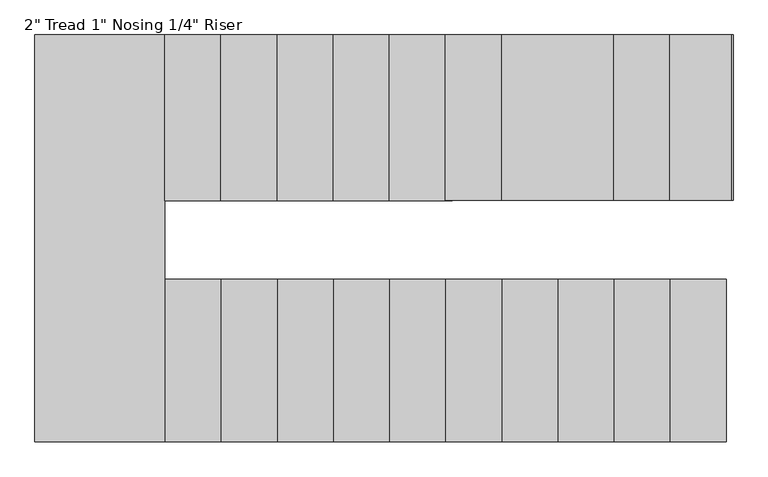
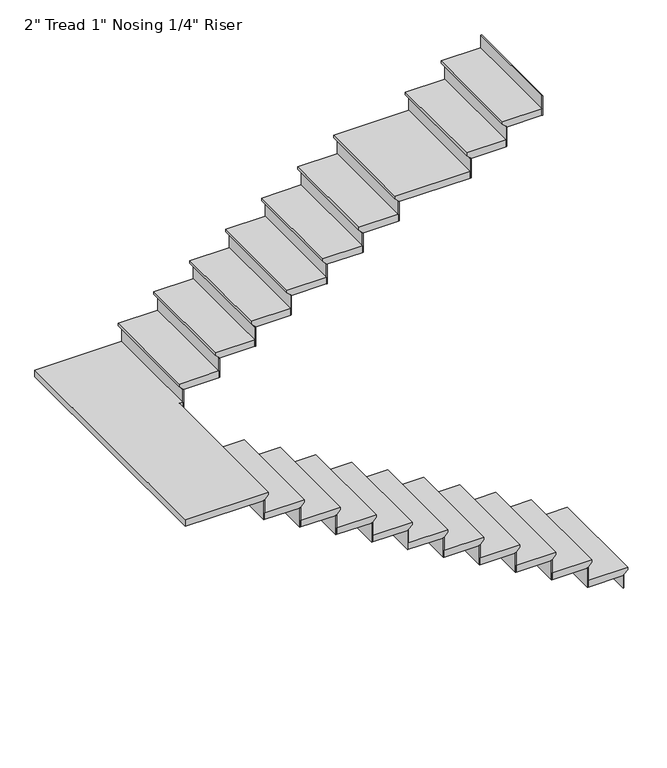
"""IFC4 building model written with IfcOpenShell, lengths in millimetres: stair flight geometry."""

from ifc_helpers import new_model, si_unit, origin, place, context, project, spatial, faceted_brep, source, transform, mapped, element, save


def stair_flight_618316a1(model_context):
    return source(origin(), model_context, "Body", "Brep", [
        faceted_brep([(-3117.2664982, -7431.6600272, 3174.0928571), (-3117.2664982, -7431.6600272, 3193.1428571), (-3117.2664982, -8168.2600272, 3193.1428571), (-3117.2664982, -8168.2600272, 3174.0928571), (-3142.6664982, -7431.6600272, 3148.6928571), (-3142.6664982, -8168.2600272, 3148.6928571), (-3396.6664982, -7431.6600272, 3193.1428571), (-3396.6664982, -8168.2600272, 3193.1428571), (-3142.6664982, -8168.2600272, 3142.3428571), (-3396.6664982, -8168.2600272, 3142.3428571), (-3396.6664982, -7431.6600272, 3142.3428571), (-3142.6664982, -7431.6600272, 3142.3428571)], [[[0, 1, 2, 3]], [[4, 0, 3, 5]], [[2, 1, 6, 7]], [[8, 9, 10, 11]], [[2, 7, 9, 8, 5, 3]], [[8, 11, 4, 5]], [[6, 1, 0, 4, 11, 10]], [[7, 6, 10, 9]]]),
        faceted_brep([(-3142.6664982, -7431.6600272, 3142.3428571), (-3142.6664982, -7431.6600272, 3048.0), (-3149.0164982, -7431.6600272, 3048.0), (-3149.0164982, -7431.6600272, 3142.3428571), (-3142.6664982, -8168.2600272, 3142.3428571), (-3149.0164982, -8168.2600272, 3142.3428571), (-3149.0164982, -8168.2600272, 3048.0), (-3142.6664982, -8168.2600272, 3048.0)], [[[0, 1, 2, 3]], [[4, 5, 6, 7]], [[1, 0, 4, 7]], [[2, 1, 7, 6]], [[3, 2, 6, 5]], [[0, 3, 5, 4]]]),
        faceted_brep([(-3396.6664982, -7431.6600272, 3287.4857143), (-3396.6664982, -7431.6600272, 3142.3428571), (-3403.0164982, -7431.6600272, 3142.3428571), (-3403.0164982, -7431.6600272, 3287.4857143), (-3396.6664982, -8168.2600272, 3287.4857143), (-3403.0164982, -8168.2600272, 3287.4857143), (-3403.0164982, -8168.2600272, 3142.3428571), (-3396.6664982, -8168.2600272, 3142.3428571)], [[[0, 1, 2, 3]], [[4, 5, 6, 7]], [[1, 0, 4, 7]], [[2, 1, 7, 6]], [[3, 2, 6, 5]], [[0, 3, 5, 4]]]),
        faceted_brep([(-3371.2664982, -8168.2600272, 3338.2857143), (-3371.2664982, -7431.6600272, 3338.2857143), (-3650.6664982, -7431.6600272, 3338.2857143), (-3650.6664982, -8168.2600272, 3338.2857143), (-3396.6664982, -8168.2600272, 3287.4857143), (-3650.6664982, -8168.2600272, 3287.4857143), (-3650.6664982, -7431.6600272, 3287.4857143), (-3396.6664982, -7431.6600272, 3287.4857143), (-3396.6664982, -8168.2600272, 3293.8357143), (-3371.2664982, -8168.2600272, 3319.2357143), (-3396.6664982, -7431.6600272, 3293.8357143), (-3371.2664982, -7431.6600272, 3319.2357143)], [[[0, 1, 2, 3]], [[4, 5, 6, 7]], [[0, 3, 5, 4, 8, 9]], [[4, 7, 10, 8]], [[2, 1, 11, 10, 7, 6]], [[3, 2, 6, 5]], [[11, 1, 0, 9]], [[10, 11, 9, 8]]]),
        faceted_brep([(-3650.6664982, -7431.6600272, 3432.6285714), (-3650.6664982, -7431.6600272, 3287.4857143), (-3657.0164982, -7431.6600272, 3287.4857143), (-3657.0164982, -7431.6600272, 3432.6285714), (-3650.6664982, -8168.2600272, 3432.6285714), (-3657.0164982, -8168.2600272, 3432.6285714), (-3657.0164982, -8168.2600272, 3287.4857143), (-3650.6664982, -8168.2600272, 3287.4857143)], [[[0, 1, 2, 3]], [[4, 5, 6, 7]], [[1, 0, 4, 7]], [[2, 1, 7, 6]], [[3, 2, 6, 5]], [[0, 3, 5, 4]]]),
        faceted_brep([(-3625.2664982, -8168.2600272, 3483.4285714), (-3625.2664982, -7431.6600272, 3483.4285714), (-3904.6664982, -7431.6600272, 3483.4285714), (-3904.6664982, -8168.2600272, 3483.4285714), (-3650.6664982, -8168.2600272, 3432.6285714), (-3904.6664982, -8168.2600272, 3432.6285714), (-3904.6664982, -7431.6600272, 3432.6285714), (-3650.6664982, -7431.6600272, 3432.6285714), (-3650.6664982, -8168.2600272, 3438.9785714), (-3625.2664982, -8168.2600272, 3464.3785714), (-3650.6664982, -7431.6600272, 3438.9785714), (-3625.2664982, -7431.6600272, 3464.3785714)], [[[0, 1, 2, 3]], [[4, 5, 6, 7]], [[0, 3, 5, 4, 8, 9]], [[4, 7, 10, 8]], [[2, 1, 11, 10, 7, 6]], [[3, 2, 6, 5]], [[11, 1, 0, 9]], [[10, 11, 9, 8]]]),
        faceted_brep([(-3904.6664982, -7431.6600272, 3577.7714286), (-3904.6664982, -7431.6600272, 3432.6285714), (-3911.0164982, -7431.6600272, 3432.6285714), (-3911.0164982, -7431.6600272, 3577.7714286), (-3904.6664982, -8168.2600272, 3577.7714286), (-3911.0164982, -8168.2600272, 3577.7714286), (-3911.0164982, -8168.2600272, 3432.6285714), (-3904.6664982, -8168.2600272, 3432.6285714)], [[[0, 1, 2, 3]], [[4, 5, 6, 7]], [[1, 0, 4, 7]], [[2, 1, 7, 6]], [[3, 2, 6, 5]], [[0, 3, 5, 4]]]),
        faceted_brep([(-3879.2664982, -8168.2600272, 3628.5714286), (-3879.2664982, -7431.6600272, 3628.5714286), (-4158.6664982, -7431.6600272, 3628.5714286), (-4158.6664982, -8168.2600272, 3628.5714286), (-3904.6664982, -8168.2600272, 3577.7714286), (-4158.6664982, -8168.2600272, 3577.7714286), (-4158.6664982, -7431.6600272, 3577.7714286), (-3904.6664982, -7431.6600272, 3577.7714286), (-3904.6664982, -8168.2600272, 3584.1214286), (-3879.2664982, -8168.2600272, 3609.5214286), (-3904.6664982, -7431.6600272, 3584.1214286), (-3879.2664982, -7431.6600272, 3609.5214286)], [[[0, 1, 2, 3]], [[4, 5, 6, 7]], [[0, 3, 5, 4, 8, 9]], [[4, 7, 10, 8]], [[2, 1, 11, 10, 7, 6]], [[3, 2, 6, 5]], [[11, 1, 0, 9]], [[10, 11, 9, 8]]]),
        faceted_brep([(-4158.6664982, -7431.6600272, 3722.9142857), (-4158.6664982, -7431.6600272, 3577.7714286), (-4165.0164982, -7431.6600272, 3577.7714286), (-4165.0164982, -7431.6600272, 3722.9142857), (-4158.6664982, -8168.2600272, 3722.9142857), (-4165.0164982, -8168.2600272, 3722.9142857), (-4165.0164982, -8168.2600272, 3577.7714286), (-4158.6664982, -8168.2600272, 3577.7714286)], [[[0, 1, 2, 3]], [[4, 5, 6, 7]], [[1, 0, 4, 7]], [[2, 1, 7, 6]], [[3, 2, 6, 5]], [[0, 3, 5, 4]]]),
        faceted_brep([(-4133.2664982, -8168.2600272, 3773.7142857), (-4133.2664982, -7431.6600272, 3773.7142857), (-4412.6664982, -7431.6600272, 3773.7142857), (-4412.6664982, -8168.2600272, 3773.7142857), (-4158.6664982, -8168.2600272, 3722.9142857), (-4412.6664982, -8168.2600272, 3722.9142857), (-4412.6664982, -7431.6600272, 3722.9142857), (-4158.6664982, -7431.6600272, 3722.9142857), (-4158.6664982, -8168.2600272, 3729.2642857), (-4133.2664982, -8168.2600272, 3754.6642857), (-4158.6664982, -7431.6600272, 3729.2642857), (-4133.2664982, -7431.6600272, 3754.6642857)], [[[0, 1, 2, 3]], [[4, 5, 6, 7]], [[0, 3, 5, 4, 8, 9]], [[4, 7, 10, 8]], [[2, 1, 11, 10, 7, 6]], [[3, 2, 6, 5]], [[11, 1, 0, 9]], [[10, 11, 9, 8]]]),
        faceted_brep([(-4412.6664982, -7431.6600272, 3868.0571429), (-4412.6664982, -7431.6600272, 3722.9142857), (-4419.0164982, -7431.6600272, 3722.9142857), (-4419.0164982, -7431.6600272, 3868.0571429), (-4412.6664982, -8168.2600272, 3868.0571429), (-4419.0164982, -8168.2600272, 3868.0571429), (-4419.0164982, -8168.2600272, 3722.9142857), (-4412.6664982, -8168.2600272, 3722.9142857)], [[[0, 1, 2, 3]], [[4, 5, 6, 7]], [[1, 0, 4, 7]], [[2, 1, 7, 6]], [[3, 2, 6, 5]], [[0, 3, 5, 4]]]),
        faceted_brep([(-4387.2664982, -8168.2600272, 3918.8571429), (-4387.2664982, -7431.6600272, 3918.8571429), (-4666.6664982, -7431.6600272, 3918.8571429), (-4666.6664982, -8168.2600272, 3918.8571429), (-4412.6664982, -8168.2600272, 3868.0571429), (-4666.6664982, -8168.2600272, 3868.0571429), (-4666.6664982, -7431.6600272, 3868.0571429), (-4412.6664982, -7431.6600272, 3868.0571429), (-4412.6664982, -8168.2600272, 3874.4071429), (-4387.2664982, -8168.2600272, 3899.8071429), (-4412.6664982, -7431.6600272, 3874.4071429), (-4387.2664982, -7431.6600272, 3899.8071429)], [[[0, 1, 2, 3]], [[4, 5, 6, 7]], [[0, 3, 5, 4, 8, 9]], [[4, 7, 10, 8]], [[2, 1, 11, 10, 7, 6]], [[3, 2, 6, 5]], [[11, 1, 0, 9]], [[10, 11, 9, 8]]]),
        faceted_brep([(-4666.6664982, -7431.6600272, 4013.2), (-4666.6664982, -7431.6600272, 3868.0571429), (-4673.0164982, -7431.6600272, 3868.0571429), (-4673.0164982, -7431.6600272, 4013.2), (-4666.6664982, -8168.2600272, 4013.2), (-4673.0164982, -8168.2600272, 4013.2), (-4673.0164982, -8168.2600272, 3868.0571429), (-4666.6664982, -8168.2600272, 3868.0571429)], [[[0, 1, 2, 3]], [[4, 5, 6, 7]], [[1, 0, 4, 7]], [[2, 1, 7, 6]], [[3, 2, 6, 5]], [[0, 3, 5, 4]]]),
        faceted_brep([(-4641.2664982, -8168.2600272, 4064.0), (-4641.2664982, -7431.6600272, 4064.0), (-4920.6664982, -7431.6600272, 4064.0), (-4920.6664982, -8168.2600272, 4064.0), (-4666.6664982, -8168.2600272, 4013.2), (-4920.6664982, -8168.2600272, 4013.2), (-4920.6664982, -7431.6600272, 4013.2), (-4666.6664982, -7431.6600272, 4013.2), (-4666.6664982, -8168.2600272, 4019.55), (-4641.2664982, -8168.2600272, 4044.95), (-4666.6664982, -7431.6600272, 4019.55), (-4641.2664982, -7431.6600272, 4044.95)], [[[0, 1, 2, 3]], [[4, 5, 6, 7]], [[0, 3, 5, 4, 8, 9]], [[4, 7, 10, 8]], [[2, 1, 11, 10, 7, 6]], [[3, 2, 6, 5]], [[11, 1, 0, 9]], [[10, 11, 9, 8]]]),
        faceted_brep([(-4920.6664982, -7431.6600272, 4158.3428571), (-4920.6664982, -7431.6600272, 4013.2), (-4927.0164982, -7431.6600272, 4013.2), (-4927.0164982, -7431.6600272, 4158.3428571), (-4920.6664982, -8168.2600272, 4158.3428571), (-4927.0164982, -8168.2600272, 4158.3428571), (-4927.0164982, -8168.2600272, 4013.2), (-4920.6664982, -8168.2600272, 4013.2)], [[[0, 1, 2, 3]], [[4, 5, 6, 7]], [[1, 0, 4, 7]], [[2, 1, 7, 6]], [[3, 2, 6, 5]], [[0, 3, 5, 4]]]),
        faceted_brep([(-4895.2664982, -8168.2600272, 4209.1428571), (-4895.2664982, -7431.6600272, 4209.1428571), (-5174.6664982, -7431.6600272, 4209.1428571), (-5174.6664982, -8168.2600272, 4209.1428571), (-4920.6664982, -8168.2600272, 4158.3428571), (-5174.6664982, -8168.2600272, 4158.3428571), (-5174.6664982, -7431.6600272, 4158.3428571), (-4920.6664982, -7431.6600272, 4158.3428571), (-4920.6664982, -8168.2600272, 4164.6928571), (-4895.2664982, -8168.2600272, 4190.0928571), (-4920.6664982, -7431.6600272, 4164.6928571), (-4895.2664982, -7431.6600272, 4190.0928571)], [[[0, 1, 2, 3]], [[4, 5, 6, 7]], [[0, 3, 5, 4, 8, 9]], [[4, 7, 10, 8]], [[2, 1, 11, 10, 7, 6]], [[3, 2, 6, 5]], [[11, 1, 0, 9]], [[10, 11, 9, 8]]]),
        faceted_brep([(-5174.6664982, -7431.6600272, 4303.4857143), (-5174.6664982, -7431.6600272, 4158.3428571), (-5181.0164982, -7431.6600272, 4158.3428571), (-5181.0164982, -7431.6600272, 4303.4857143), (-5174.6664982, -8168.2600272, 4303.4857143), (-5181.0164982, -8168.2600272, 4303.4857143), (-5181.0164982, -8168.2600272, 4158.3428571), (-5174.6664982, -8168.2600272, 4158.3428571)], [[[0, 1, 2, 3]], [[4, 5, 6, 7]], [[1, 0, 4, 7]], [[2, 1, 7, 6]], [[3, 2, 6, 5]], [[0, 3, 5, 4]]]),
        faceted_brep([(-5149.2664982, -8168.2600272, 4354.2857143), (-5149.2664982, -7431.6600272, 4354.2857143), (-5428.6664982, -7431.6600272, 4354.2857143), (-5428.6664982, -8168.2600272, 4354.2857143), (-5174.6664982, -8168.2600272, 4303.4857143), (-5428.6664982, -8168.2600272, 4303.4857143), (-5428.6664982, -7431.6600272, 4303.4857143), (-5174.6664982, -7431.6600272, 4303.4857143), (-5174.6664982, -8168.2600272, 4309.8357143), (-5149.2664982, -8168.2600272, 4335.2357143), (-5174.6664982, -7431.6600272, 4309.8357143), (-5149.2664982, -7431.6600272, 4335.2357143)], [[[0, 1, 2, 3]], [[4, 5, 6, 7]], [[0, 3, 5, 4, 8, 9]], [[4, 7, 10, 8]], [[2, 1, 11, 10, 7, 6]], [[3, 2, 6, 5]], [[11, 1, 0, 9]], [[10, 11, 9, 8]]]),
        faceted_brep([(-5428.6664982, -7431.6600272, 4448.6285714), (-5428.6664982, -7431.6600272, 4303.4857143), (-5435.0164982, -7431.6600272, 4303.4857143), (-5435.0164982, -7431.6600272, 4448.6285714), (-5428.6664982, -8168.2600272, 4448.6285714), (-5435.0164982, -8168.2600272, 4448.6285714), (-5435.0164982, -8168.2600272, 4303.4857143), (-5428.6664982, -8168.2600272, 4303.4857143)], [[[0, 1, 2, 3]], [[4, 5, 6, 7]], [[1, 0, 4, 7]], [[2, 1, 7, 6]], [[3, 2, 6, 5]], [[0, 3, 5, 4]]]),
        faceted_brep([(-5403.2664982, -8168.2600272, 4499.4285714), (-5403.2664982, -7431.6600272, 4499.4285714), (-5682.6664982, -7431.6600272, 4499.4285714), (-5682.6664982, -8168.2600272, 4499.4285714), (-5428.6664982, -8168.2600272, 4448.6285714), (-5682.6664982, -8168.2600272, 4448.6285714), (-5682.6664982, -7431.6600272, 4448.6285714), (-5428.6664982, -7431.6600272, 4448.6285714), (-5428.6664982, -8168.2600272, 4454.9785714), (-5403.2664982, -8168.2600272, 4480.3785714), (-5428.6664982, -7431.6600272, 4454.9785714), (-5403.2664982, -7431.6600272, 4480.3785714)], [[[0, 1, 2, 3]], [[4, 5, 6, 7]], [[0, 3, 5, 4, 8, 9]], [[4, 7, 10, 8]], [[2, 1, 11, 10, 7, 6]], [[3, 2, 6, 5]], [[11, 1, 0, 9]], [[10, 11, 9, 8]]]),
        faceted_brep([(-5682.6664982, -7431.6600272, 4593.7714286), (-5682.6664982, -7431.6600272, 4448.6285714), (-5689.0164982, -7431.6600272, 4448.6285714), (-5689.0164982, -7431.6600272, 4593.7714286), (-5682.6664982, -8168.2600272, 4593.7714286), (-5689.0164982, -8168.2600272, 4593.7714286), (-5689.0164982, -8168.2600272, 4448.6285714), (-5682.6664982, -8168.2600272, 4448.6285714)], [[[0, 1, 2, 3]], [[4, 5, 6, 7]], [[1, 0, 4, 7]], [[2, 1, 7, 6]], [[3, 2, 6, 5]], [[0, 3, 5, 4]]]),
        faceted_brep([(-5631.8664982, -6326.7600272, 4644.5714286), (-6245.2108866, -6326.7600272, 4644.5714286), (-6245.2108866, -8168.2600272, 4644.5714286), (-5657.2664982, -8168.2600272, 4644.5714286), (-5657.2664982, -7076.0600272, 4644.5714286), (-5631.8664982, -7076.0600272, 4644.5714286), (-6245.2108866, -6326.7600272, 4593.7714286), (-5631.8664982, -6326.7600272, 4593.7714286), (-5631.8664982, -7076.0600272, 4593.7714286), (-5657.2664982, -7076.0600272, 4593.7714286), (-5657.2664982, -7431.6600272, 4593.7714286), (-5682.6664982, -7431.6600272, 4593.7714286), (-5682.6664982, -8168.2600272, 4593.7714286), (-6245.2108866, -8168.2600272, 4593.7714286), (-5682.6664982, -8168.2600272, 4600.1214286), (-5657.2664982, -8168.2600272, 4625.5214286), (-5682.6664982, -7431.6600272, 4600.1214286), (-5657.2664982, -7431.6600272, 4625.5214286)], [[[0, 1, 2, 3, 4, 5]], [[6, 7, 8, 9, 10, 11, 12, 13]], [[1, 0, 7, 6]], [[2, 1, 6, 13]], [[3, 2, 13, 12, 14, 15]], [[12, 11, 16, 14]], [[11, 10, 17, 16]], [[4, 3, 15, 17, 10, 9]], [[5, 4, 9, 8]], [[0, 5, 8, 7]], [[15, 14, 16, 17]]]),
        faceted_brep([(-5631.8664982, -7076.0600272, 4738.9142857), (-5631.8664982, -7076.0600272, 4593.7714286), (-5625.5164982, -7076.0600272, 4593.7714286), (-5625.5164982, -7076.0600272, 4738.9142857), (-5631.8664982, -6326.7600272, 4738.9142857), (-5625.5164982, -6326.7600272, 4738.9142857), (-5625.5164982, -6326.7600272, 4593.7714286), (-5631.8664982, -6326.7600272, 4593.7714286)], [[[0, 1, 2, 3]], [[4, 5, 6, 7]], [[1, 0, 4, 7]], [[2, 1, 7, 6]], [[3, 2, 6, 5]], [[0, 3, 5, 4]]]),
        faceted_brep([(-5657.2664982, -6326.7600272, 4789.7142857), (-5657.2664982, -7076.0600272, 4789.7142857), (-5377.8664982, -7076.0600272, 4789.7142857), (-5377.8664982, -6326.7600272, 4789.7142857), (-5631.8664982, -6326.7600272, 4738.9142857), (-5377.8664982, -6326.7600272, 4738.9142857), (-5377.8664982, -7076.0600272, 4738.9142857), (-5631.8664982, -7076.0600272, 4738.9142857), (-5631.8664982, -6326.7600272, 4745.2642857), (-5657.2664982, -6326.7600272, 4770.6642857), (-5631.8664982, -7076.0600272, 4745.2642857), (-5657.2664982, -7076.0600272, 4770.6642857)], [[[0, 1, 2, 3]], [[4, 5, 6, 7]], [[0, 3, 5, 4, 8, 9]], [[4, 7, 10, 8]], [[2, 1, 11, 10, 7, 6]], [[3, 2, 6, 5]], [[11, 1, 0, 9]], [[10, 11, 9, 8]]]),
        faceted_brep([(-5377.8664982, -7076.0600272, 4884.0571429), (-5377.8664982, -7076.0600272, 4738.9142857), (-5371.5164982, -7076.0600272, 4738.9142857), (-5371.5164982, -7076.0600272, 4884.0571429), (-5377.8664982, -6326.7600272, 4884.0571429), (-5371.5164982, -6326.7600272, 4884.0571429), (-5371.5164982, -6326.7600272, 4738.9142857), (-5377.8664982, -6326.7600272, 4738.9142857)], [[[0, 1, 2, 3]], [[4, 5, 6, 7]], [[1, 0, 4, 7]], [[2, 1, 7, 6]], [[3, 2, 6, 5]], [[0, 3, 5, 4]]]),
        faceted_brep([(-5403.2664982, -6326.7600272, 4934.8571429), (-5403.2664982, -7076.0600272, 4934.8571429), (-5123.8664982, -7076.0600272, 4934.8571429), (-5123.8664982, -6326.7600272, 4934.8571429), (-5377.8664982, -6326.7600272, 4884.0571429), (-5123.8664982, -6326.7600272, 4884.0571429), (-5123.8664982, -7076.0600272, 4884.0571429), (-5377.8664982, -7076.0600272, 4884.0571429), (-5377.8664982, -6326.7600272, 4890.4071429), (-5403.2664982, -6326.7600272, 4915.8071429), (-5377.8664982, -7076.0600272, 4890.4071429), (-5403.2664982, -7076.0600272, 4915.8071429)], [[[0, 1, 2, 3]], [[4, 5, 6, 7]], [[0, 3, 5, 4, 8, 9]], [[4, 7, 10, 8]], [[2, 1, 11, 10, 7, 6]], [[3, 2, 6, 5]], [[11, 1, 0, 9]], [[10, 11, 9, 8]]]),
        faceted_brep([(-5123.8664982, -7076.0600272, 5029.2), (-5123.8664982, -7076.0600272, 4884.0571429), (-5117.5164982, -7076.0600272, 4884.0571429), (-5117.5164982, -7076.0600272, 5029.2), (-5123.8664982, -6326.7600272, 5029.2), (-5117.5164982, -6326.7600272, 5029.2), (-5117.5164982, -6326.7600272, 4884.0571429), (-5123.8664982, -6326.7600272, 4884.0571429)], [[[0, 1, 2, 3]], [[4, 5, 6, 7]], [[1, 0, 4, 7]], [[2, 1, 7, 6]], [[3, 2, 6, 5]], [[0, 3, 5, 4]]]),
        faceted_brep([(-5149.2664982, -6326.7600272, 5080.0), (-5149.2664982, -7076.0600272, 5080.0), (-4869.8664982, -7076.0600272, 5080.0), (-4869.8664982, -6326.7600272, 5080.0), (-5123.8664982, -6326.7600272, 5029.2), (-4869.8664982, -6326.7600272, 5029.2), (-4869.8664982, -7076.0600272, 5029.2), (-5123.8664982, -7076.0600272, 5029.2), (-5123.8664982, -6326.7600272, 5035.55), (-5149.2664982, -6326.7600272, 5060.95), (-5123.8664982, -7076.0600272, 5035.55), (-5149.2664982, -7076.0600272, 5060.95)], [[[0, 1, 2, 3]], [[4, 5, 6, 7]], [[0, 3, 5, 4, 8, 9]], [[4, 7, 10, 8]], [[2, 1, 11, 10, 7, 6]], [[3, 2, 6, 5]], [[11, 1, 0, 9]], [[10, 11, 9, 8]]]),
        faceted_brep([(-4869.8664982, -7076.0600272, 5174.3428571), (-4869.8664982, -7076.0600272, 5029.2), (-4863.5164982, -7076.0600272, 5029.2), (-4863.5164982, -7076.0600272, 5174.3428571), (-4869.8664982, -6326.7600272, 5174.3428571), (-4863.5164982, -6326.7600272, 5174.3428571), (-4863.5164982, -6326.7600272, 5029.2), (-4869.8664982, -6326.7600272, 5029.2)], [[[0, 1, 2, 3]], [[4, 5, 6, 7]], [[1, 0, 4, 7]], [[2, 1, 7, 6]], [[3, 2, 6, 5]], [[0, 3, 5, 4]]]),
        faceted_brep([(-4895.2664982, -6326.7600272, 5225.1428571), (-4895.2664982, -7076.0600272, 5225.1428571), (-4615.8664982, -7076.0600272, 5225.1428571), (-4615.8664982, -6326.7600272, 5225.1428571), (-4869.8664982, -6326.7600272, 5174.3428571), (-4615.8664982, -6326.7600272, 5174.3428571), (-4615.8664982, -7076.0600272, 5174.3428571), (-4869.8664982, -7076.0600272, 5174.3428571), (-4869.8664982, -6326.7600272, 5180.6928571), (-4895.2664982, -6326.7600272, 5206.0928571), (-4869.8664982, -7076.0600272, 5180.6928571), (-4895.2664982, -7076.0600272, 5206.0928571)], [[[0, 1, 2, 3]], [[4, 5, 6, 7]], [[0, 3, 5, 4, 8, 9]], [[4, 7, 10, 8]], [[2, 1, 11, 10, 7, 6]], [[3, 2, 6, 5]], [[11, 1, 0, 9]], [[10, 11, 9, 8]]]),
        faceted_brep([(-4615.8664982, -7076.0600272, 5319.4857143), (-4615.8664982, -7076.0600272, 5174.3428571), (-4609.5164982, -7076.0600272, 5174.3428571), (-4609.5164982, -7076.0600272, 5319.4857143), (-4615.8664982, -6326.7600272, 5319.4857143), (-4609.5164982, -6326.7600272, 5319.4857143), (-4609.5164982, -6326.7600272, 5174.3428571), (-4615.8664982, -6326.7600272, 5174.3428571)], [[[0, 1, 2, 3]], [[4, 5, 6, 7]], [[1, 0, 4, 7]], [[2, 1, 7, 6]], [[3, 2, 6, 5]], [[0, 3, 5, 4]]]),
        faceted_brep([(-4641.2664982, -6326.7600272, 5370.2857143), (-4641.2664982, -7076.0600272, 5370.2857143), (-4361.8664982, -7076.0600272, 5370.2857143), (-4361.8664982, -6326.7600272, 5370.2857143), (-4615.8664982, -6326.7600272, 5319.4857143), (-4361.8664982, -6326.7600272, 5319.4857143), (-4361.8664982, -7076.0600272, 5319.4857143), (-4615.8664982, -7076.0600272, 5319.4857143), (-4615.8664982, -6326.7600272, 5325.8357143), (-4641.2664982, -6326.7600272, 5351.2357143), (-4615.8664982, -7076.0600272, 5325.8357143), (-4641.2664982, -7076.0600272, 5351.2357143)], [[[0, 1, 2, 3]], [[4, 5, 6, 7]], [[0, 3, 5, 4, 8, 9]], [[4, 7, 10, 8]], [[2, 1, 11, 10, 7, 6]], [[3, 2, 6, 5]], [[11, 1, 0, 9]], [[10, 11, 9, 8]]]),
        faceted_brep([(-4361.8664982, -7076.0600272, 5464.6285714), (-4361.8664982, -7076.0600272, 5319.4857143), (-4355.5164982, -7076.0600272, 5319.4857143), (-4355.5164982, -7076.0600272, 5464.6285714), (-4361.8664982, -6326.7600272, 5464.6285714), (-4355.5164982, -6326.7600272, 5464.6285714), (-4355.5164982, -6326.7600272, 5319.4857143), (-4361.8664982, -6326.7600272, 5319.4857143)], [[[0, 1, 2, 3]], [[4, 5, 6, 7]], [[1, 0, 4, 7]], [[2, 1, 7, 6]], [[3, 2, 6, 5]], [[0, 3, 5, 4]]]),
        faceted_brep([(-4387.2664982, -6326.7600272, 5515.4285714), (-4387.2664982, -7076.0600272, 5515.4285714), (-4107.8664982, -7076.0600272, 5515.4285714), (-4107.8664982, -6326.7600272, 5515.4285714), (-4361.8664982, -6326.7600272, 5464.6285714), (-4107.8664982, -6326.7600272, 5464.6285714), (-4107.8664982, -7076.0600272, 5464.6285714), (-4361.8664982, -7076.0600272, 5464.6285714), (-4361.8664982, -6326.7600272, 5470.9785714), (-4387.2664982, -6326.7600272, 5496.3785714), (-4361.8664982, -7076.0600272, 5470.9785714), (-4387.2664982, -7076.0600272, 5496.3785714)], [[[0, 1, 2, 3]], [[4, 5, 6, 7]], [[0, 3, 5, 4, 8, 9]], [[4, 7, 10, 8]], [[2, 1, 11, 10, 7, 6]], [[3, 2, 6, 5]], [[11, 1, 0, 9]], [[10, 11, 9, 8]]]),
        faceted_brep([(-4107.8664982, -7076.0600272, 5609.7714286), (-4107.8664982, -7076.0600272, 5464.6285714), (-4101.5164982, -7076.0600272, 5464.6285714), (-4101.5164982, -7076.0600272, 5609.7714286), (-4107.8664982, -6326.7600272, 5609.7714286), (-4101.5164982, -6326.7600272, 5609.7714286), (-4101.5164982, -6326.7600272, 5464.6285714), (-4107.8664982, -6326.7600272, 5464.6285714)], [[[0, 1, 2, 3]], [[4, 5, 6, 7]], [[1, 0, 4, 7]], [[2, 1, 7, 6]], [[3, 2, 6, 5]], [[0, 3, 5, 4]]]),
        faceted_brep([(-4133.2664982, -6326.7600272, 5660.5714286), (-4133.2664982, -7076.0600272, 5660.5714286), (-3599.8664982, -7076.0600272, 5660.5714286), (-3599.8664982, -6326.7600272, 5660.5714286), (-4107.8664982, -6326.7600272, 5609.7714286), (-3599.8664982, -6326.7600272, 5609.7714286), (-3599.8664982, -7076.0600272, 5609.7714286), (-4107.8664982, -7076.0600272, 5609.7714286), (-4107.8664982, -6326.7600272, 5616.1214286), (-4133.2664982, -6326.7600272, 5641.5214286), (-4107.8664982, -7076.0600272, 5616.1214286), (-4133.2664982, -7076.0600272, 5641.5214286)], [[[0, 1, 2, 3]], [[4, 5, 6, 7]], [[0, 3, 5, 4, 8, 9]], [[4, 7, 10, 8]], [[2, 1, 11, 10, 7, 6]], [[3, 2, 6, 5]], [[11, 1, 0, 9]], [[10, 11, 9, 8]]]),
        faceted_brep([(-3599.8664982, -7076.0600272, 5754.9142857), (-3599.8664982, -7076.0600272, 5609.7714286), (-3593.5164982, -7076.0600272, 5609.7714286), (-3593.5164982, -7076.0600272, 5754.9142857), (-3599.8664982, -6326.7600272, 5754.9142857), (-3593.5164982, -6326.7600272, 5754.9142857), (-3593.5164982, -6326.7600272, 5609.7714286), (-3599.8664982, -6326.7600272, 5609.7714286)], [[[0, 1, 2, 3]], [[4, 5, 6, 7]], [[1, 0, 4, 7]], [[2, 1, 7, 6]], [[3, 2, 6, 5]], [[0, 3, 5, 4]]]),
        faceted_brep([(-3625.2664982, -6326.7600272, 5805.7142857), (-3625.2664982, -7076.0600272, 5805.7142857), (-3345.8664982, -7076.0600272, 5805.7142857), (-3345.8664982, -6326.7600272, 5805.7142857), (-3599.8664982, -6326.7600272, 5754.9142857), (-3345.8664982, -6326.7600272, 5754.9142857), (-3345.8664982, -7076.0600272, 5754.9142857), (-3599.8664982, -7076.0600272, 5754.9142857), (-3599.8664982, -6326.7600272, 5761.2642857), (-3625.2664982, -6326.7600272, 5786.6642857), (-3599.8664982, -7076.0600272, 5761.2642857), (-3625.2664982, -7076.0600272, 5786.6642857)], [[[0, 1, 2, 3]], [[4, 5, 6, 7]], [[0, 3, 5, 4, 8, 9]], [[4, 7, 10, 8]], [[2, 1, 11, 10, 7, 6]], [[3, 2, 6, 5]], [[11, 1, 0, 9]], [[10, 11, 9, 8]]]),
        faceted_brep([(-3345.8664982, -7076.0600272, 5900.0571429), (-3345.8664982, -7076.0600272, 5754.9142857), (-3339.5164982, -7076.0600272, 5754.9142857), (-3339.5164982, -7076.0600272, 5900.0571429), (-3345.8664982, -6326.7600272, 5900.0571429), (-3339.5164982, -6326.7600272, 5900.0571429), (-3339.5164982, -6326.7600272, 5754.9142857), (-3345.8664982, -6326.7600272, 5754.9142857)], [[[0, 1, 2, 3]], [[4, 5, 6, 7]], [[1, 0, 4, 7]], [[2, 1, 7, 6]], [[3, 2, 6, 5]], [[0, 3, 5, 4]]]),
        faceted_brep([(-3091.8664982, -7076.0600272, 6045.2), (-3091.8664982, -7076.0600272, 5900.0571429), (-3085.5164982, -7076.0600272, 5900.0571429), (-3085.5164982, -7076.0600272, 6045.2), (-3091.8664982, -6326.7600272, 6045.2), (-3085.5164982, -6326.7600272, 6045.2), (-3085.5164982, -6326.7600272, 5900.0571429), (-3091.8664982, -6326.7600272, 5900.0571429)], [[[0, 1, 2, 3]], [[4, 5, 6, 7]], [[1, 0, 4, 7]], [[2, 1, 7, 6]], [[3, 2, 6, 5]], [[0, 3, 5, 4]]]),
        faceted_brep([(-3371.2664982, -6326.7600272, 5950.8571429), (-3371.2664982, -7076.0600272, 5950.8571429), (-3091.8664982, -7076.0600272, 5950.8571429), (-3091.8664982, -6326.7600272, 5950.8571429), (-3345.8664982, -6326.7600272, 5900.0571429), (-3091.8664982, -6326.7600272, 5900.0571429), (-3091.8664982, -7076.0600272, 5900.0571429), (-3345.8664982, -7076.0600272, 5900.0571429), (-3345.8664982, -6326.7600272, 5906.4071429), (-3371.2664982, -6326.7600272, 5931.8071429), (-3345.8664982, -7076.0600272, 5906.4071429), (-3371.2664982, -7076.0600272, 5931.8071429)], [[[0, 1, 2, 3]], [[4, 5, 6, 7]], [[0, 3, 5, 4, 8, 9]], [[4, 7, 10, 8]], [[2, 1, 11, 10, 7, 6]], [[3, 2, 6, 5]], [[11, 1, 0, 9]], [[10, 11, 9, 8]]]),
    ])


if __name__ == "__main__":
    model = new_model("IFC4")
    model_context = context("Model", 3, world=origin())
    ifc_project = project(units=[si_unit("LENGTHUNIT", "METRE", prefix="MILLI")], contexts=[model_context])
    site = spatial("IfcSite", under=ifc_project)
    building = spatial("IfcBuilding", under=site)
    placement = place(None, origin())
    stair_flight_shape = stair_flight_618316a1(model_context)
    element("IfcStairFlight", 1, ObjectType="2\" Tread 1\" Nosing 1/4\" Riser", at=placement, inside=building, context=model_context, shape_type="MappedRepresentation", body=[
        mapped(stair_flight_shape, transform((0.0, 0.0, 0.0), x_axis=(1.0, 0.0, 0.0), y_axis=(0.0, 1.0, 0.0), z_axis=(0.0, 0.0, 1.0))),
    ])
    save(model, "model.ifc")
